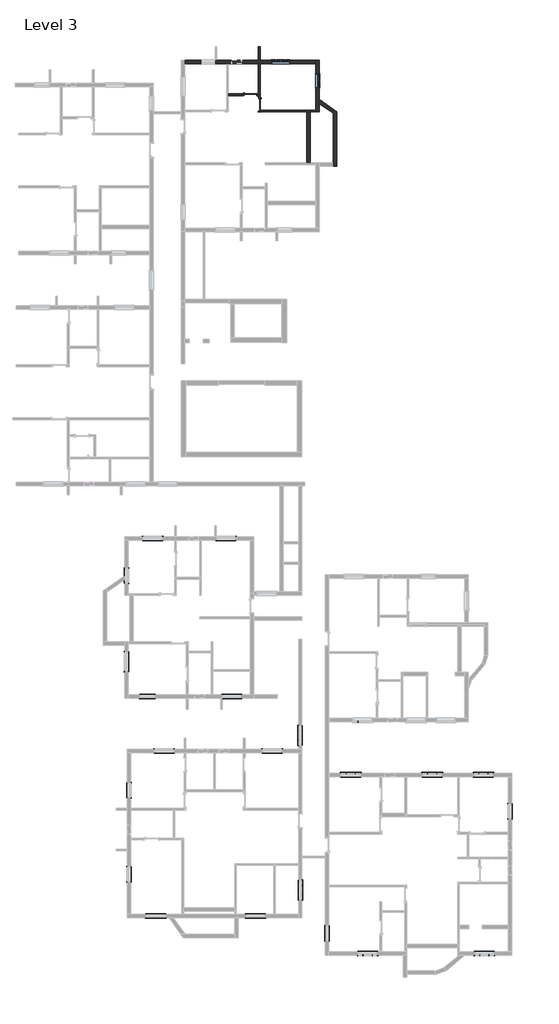
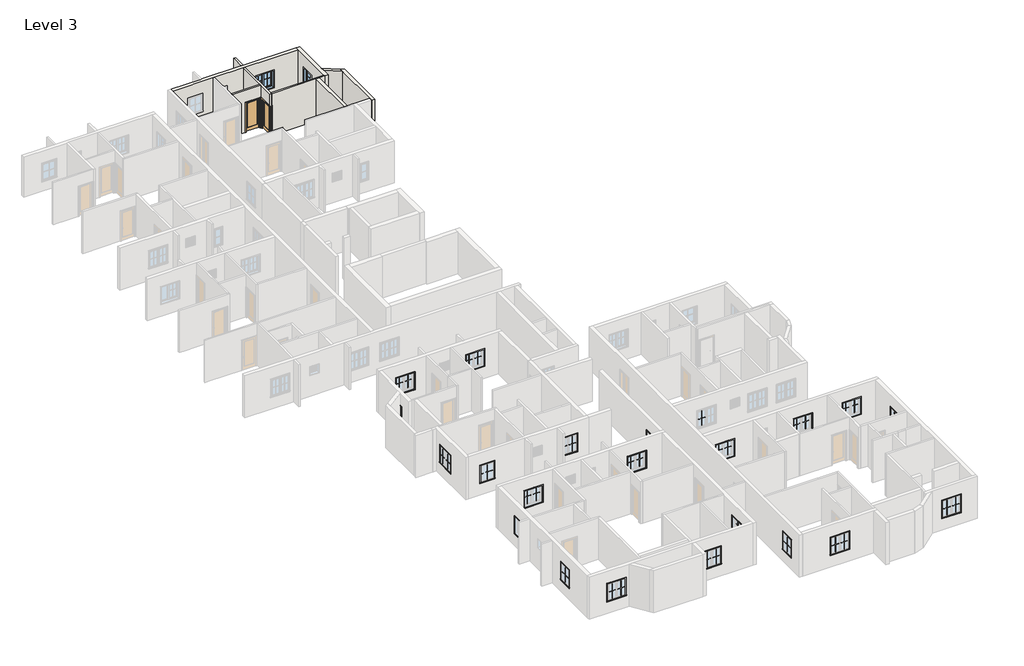
# One storey, part 6 of 7: 79 proxies, 9 walls, 2 doors, 2 windows.
"""IFC4 building model written with IfcOpenShell, lengths in millimetres."""

from ifc_helpers import new_model, si_unit, frame, origin, place, context, project, spatial, polyline, outline, extrude, faceted_brep, transform, mapped, element, save
from components import muntin_pattern_2x2_muntin_pattern_2x2_95b57395, muntin_pattern_2x2_muntin_pattern_2x2_4dfeb3f3, muntin_pattern_2x2_muntin_pattern_2x2_e852a7e4, trim_window_exterior_flat_with_sill_e4b28ec3, trim_window_exterior_flat_with_sill_7cfdd449, trim_window_interior_flat_picture_frame_39ff4276, trim_window_interior_flat_picture_frame_f1e0b15b, door_3c6ab76a, window_272f20d6, window_casement_double_4_x_4_af3140d2

model = new_model("IFC4")

# Units and contexts
model_context = context("Model", 3, world=origin())
ifc_project = project(units=[si_unit("LENGTHUNIT", "METRE", prefix="MILLI")], contexts=[model_context])

# Site, building, storey
site = spatial("IfcSite", under=ifc_project)
building = spatial("IfcBuilding", under=site)
storey = spatial("IfcBuildingStorey", under=building, Name="Level 3", Elevation=3200.4)

# Proxies
placement = place(None, origin())
muntin_pattern_2x2_muntin_pattern_2x2_shape = muntin_pattern_2x2_muntin_pattern_2x2_95b57395(model_context)
element("IfcBuildingElementProxy", 1, Name="Muntin Pattern_2x2 : Muntin Pattern_2x2", ObjectType="Muntin Pattern_2x2 : Muntin Pattern_2x2", at=placement, inside=storey, context=model_context, shape_type="MappedRepresentation", body=[
    mapped(muntin_pattern_2x2_muntin_pattern_2x2_shape, transform((17627.3240531, -20041.5997229, 4184.65), x_axis=(0.0, 1.0, 0.0), y_axis=(-1.0, 0.0, 0.0), z_axis=(0.0, 0.0, 1.0))),
])
element("IfcBuildingElementProxy", 2, Name="Muntin Pattern_2x2 : Muntin Pattern_2x2", ObjectType="Muntin Pattern_2x2 : Muntin Pattern_2x2", at=placement, inside=storey, context=model_context, shape_type="MappedRepresentation", body=[
    mapped(muntin_pattern_2x2_muntin_pattern_2x2_shape, transform((5625.8240531, -28048.9497229, 4184.65), x_axis=(0.0, 1.0, 0.0), y_axis=(-1.0, 0.0, 0.0), z_axis=(0.0, 0.0, 1.0))),
])
element("IfcBuildingElementProxy", 3, Name="Muntin Pattern_2x2 : Muntin Pattern_2x2", ObjectType="Muntin Pattern_2x2 : Muntin Pattern_2x2", at=placement, inside=storey, context=model_context, shape_type="MappedRepresentation", body=[
    mapped(muntin_pattern_2x2_muntin_pattern_2x2_shape, transform((-7378.9759469, -24172.9363256, 4184.65), x_axis=(0.0, 1.0, 0.0), y_axis=(-1.0, 0.0, 0.0), z_axis=(0.0, 0.0, 1.0))),
])
element("IfcBuildingElementProxy", 4, Name="Muntin Pattern_2x2 : Muntin Pattern_2x2", ObjectType="Muntin Pattern_2x2 : Muntin Pattern_2x2", at=placement, inside=storey, context=model_context, shape_type="MappedRepresentation", body=[
    mapped(muntin_pattern_2x2_muntin_pattern_2x2_shape, transform((-7169.4259469, -18656.0038828, 4184.65), x_axis=(0.0, -1.0, 0.0), y_axis=(1.0, 0.0, 0.0), z_axis=(0.0, 0.0, 1.0))),
])
element("IfcBuildingElementProxy", 5, Name="Muntin Pattern_2x2 : Muntin Pattern_2x2", ObjectType="Muntin Pattern_2x2 : Muntin Pattern_2x2", at=placement, inside=storey, context=model_context, shape_type="MappedRepresentation", body=[
    mapped(muntin_pattern_2x2_muntin_pattern_2x2_shape, transform((-6067.7009469, -12594.9288828, 4184.65), x_axis=(-1.0, 0.0, 0.0), y_axis=(0.0, -1.0, 0.0), z_axis=(0.0, 0.0, 1.0))),
])
element("IfcBuildingElementProxy", 6, Name="Muntin Pattern_2x2 : Muntin Pattern_2x2", ObjectType="Muntin Pattern_2x2 : Muntin Pattern_2x2", at=placement, inside=storey, context=model_context, shape_type="MappedRepresentation", body=[
    mapped(muntin_pattern_2x2_muntin_pattern_2x2_shape, transform((-7334.5259469, -4559.0038828, 4184.65), x_axis=(0.0, -1.0, 0.0), y_axis=(1.0, 0.0, 0.0), z_axis=(0.0, 0.0, 1.0))),
])
muntin_pattern_2x2_muntin_pattern_2x2_2_shape = muntin_pattern_2x2_muntin_pattern_2x2_4dfeb3f3(model_context)
element("IfcBuildingElementProxy", 7, Name="Muntin Pattern_2x2 : Muntin Pattern_2x2", ObjectType="Muntin Pattern_2x2 : Muntin Pattern_2x2", at=placement, inside=storey, context=model_context, shape_type="MappedRepresentation", body=[
    mapped(muntin_pattern_2x2_muntin_pattern_2x2_2_shape, transform((6976.7865531, -17530.1747229, 4184.65), x_axis=(1.0, 0.0, 0.0), y_axis=(0.0, 1.0, 0.0), z_axis=(0.0, 0.0, 1.0))),
])
element("IfcBuildingElementProxy", 8, Name="Muntin Pattern_2x2 : Muntin Pattern_2x2", ObjectType="Muntin Pattern_2x2 : Muntin Pattern_2x2", at=placement, inside=storey, context=model_context, shape_type="MappedRepresentation", body=[
    mapped(muntin_pattern_2x2_muntin_pattern_2x2_2_shape, transform((12323.4865531, -17530.1747229, 4184.65), x_axis=(1.0, 0.0, 0.0), y_axis=(0.0, 1.0, 0.0), z_axis=(0.0, 0.0, 1.0))),
])
element("IfcBuildingElementProxy", 9, Name="Muntin Pattern_2x2 : Muntin Pattern_2x2", ObjectType="Muntin Pattern_2x2 : Muntin Pattern_2x2", at=placement, inside=storey, context=model_context, shape_type="MappedRepresentation", body=[
    mapped(muntin_pattern_2x2_muntin_pattern_2x2_2_shape, transform((15682.6365531, -17530.1747229, 4184.65), x_axis=(1.0, 0.0, 0.0), y_axis=(0.0, 1.0, 0.0), z_axis=(0.0, 0.0, 1.0))),
])
element("IfcBuildingElementProxy", 10, Name="Muntin Pattern_2x2 : Muntin Pattern_2x2", ObjectType="Muntin Pattern_2x2 : Muntin Pattern_2x2", at=placement, inside=storey, context=model_context, shape_type="MappedRepresentation", body=[
    mapped(muntin_pattern_2x2_muntin_pattern_2x2_2_shape, transform((16349.3865531, -29474.5247229, 4184.65), x_axis=(-1.0, 0.0, 0.0), y_axis=(0.0, -1.0, 0.0), z_axis=(0.0, 0.0, 1.0))),
])
element("IfcBuildingElementProxy", 11, Name="Muntin Pattern_2x2 : Muntin Pattern_2x2", ObjectType="Muntin Pattern_2x2 : Muntin Pattern_2x2", at=placement, inside=storey, context=model_context, shape_type="MappedRepresentation", body=[
    mapped(muntin_pattern_2x2_muntin_pattern_2x2_2_shape, transform((8694.4615531, -29474.5247229, 4184.65), x_axis=(-1.0, 0.0, 0.0), y_axis=(0.0, -1.0, 0.0), z_axis=(0.0, 0.0, 1.0))),
])
element("IfcBuildingElementProxy", 12, Name="Muntin Pattern_2x2 : Muntin Pattern_2x2", ObjectType="Muntin Pattern_2x2 : Muntin Pattern_2x2", at=placement, inside=storey, context=model_context, shape_type="MappedRepresentation", body=[
    mapped(muntin_pattern_2x2_muntin_pattern_2x2_2_shape, transform((4070.0740531, -24902.8163828, 4184.65), x_axis=(0.0, -1.0, 0.0), y_axis=(1.0, 0.0, 0.0), z_axis=(0.0, 0.0, 1.0))),
])
element("IfcBuildingElementProxy", 13, Name="Muntin Pattern_2x2 : Muntin Pattern_2x2", ObjectType="Muntin Pattern_2x2 : Muntin Pattern_2x2", at=placement, inside=storey, context=model_context, shape_type="MappedRepresentation", body=[
    mapped(muntin_pattern_2x2_muntin_pattern_2x2_2_shape, transform((1325.2865531, -26996.7288828, 4184.65), x_axis=(-1.0, 0.0, 0.0), y_axis=(0.0, -1.0, 0.0), z_axis=(0.0, 0.0, 1.0))),
])
element("IfcBuildingElementProxy", 14, Name="Muntin Pattern_2x2 : Muntin Pattern_2x2", ObjectType="Muntin Pattern_2x2 : Muntin Pattern_2x2", at=placement, inside=storey, context=model_context, shape_type="MappedRepresentation", body=[
    mapped(muntin_pattern_2x2_muntin_pattern_2x2_2_shape, transform((-5208.8634469, -26996.7288828, 4184.65), x_axis=(-1.0, 0.0, 0.0), y_axis=(0.0, -1.0, 0.0), z_axis=(0.0, 0.0, 1.0))),
])
element("IfcBuildingElementProxy", 15, Name="Muntin Pattern_2x2 : Muntin Pattern_2x2", ObjectType="Muntin Pattern_2x2 : Muntin Pattern_2x2", at=placement, inside=storey, context=model_context, shape_type="MappedRepresentation", body=[
    mapped(muntin_pattern_2x2_muntin_pattern_2x2_2_shape, transform((1823.7615531, -15966.7788828, 4184.65), x_axis=(1.0, 0.0, 0.0), y_axis=(0.0, 1.0, 0.0), z_axis=(0.0, 0.0, 1.0))),
])
element("IfcBuildingElementProxy", 16, Name="Muntin Pattern_2x2 : Muntin Pattern_2x2", ObjectType="Muntin Pattern_2x2 : Muntin Pattern_2x2", at=placement, inside=storey, context=model_context, shape_type="MappedRepresentation", body=[
    mapped(muntin_pattern_2x2_muntin_pattern_2x2_2_shape, transform((-5272.3634469, -15966.7788828, 4184.65), x_axis=(1.0, 0.0, 0.0), y_axis=(0.0, 1.0, 0.0), z_axis=(0.0, 0.0, 1.0))),
])
element("IfcBuildingElementProxy", 17, Name="Muntin Pattern_2x2 : Muntin Pattern_2x2", ObjectType="Muntin Pattern_2x2 : Muntin Pattern_2x2", at=placement, inside=storey, context=model_context, shape_type="MappedRepresentation", body=[
    mapped(muntin_pattern_2x2_muntin_pattern_2x2_2_shape, transform((3860.5240531, -15358.7663828, 4184.65), x_axis=(0.0, 1.0, 0.0), y_axis=(-1.0, 0.0, 0.0), z_axis=(0.0, 0.0, 1.0))),
])
element("IfcBuildingElementProxy", 18, Name="Muntin Pattern_2x2 : Muntin Pattern_2x2", ObjectType="Muntin Pattern_2x2 : Muntin Pattern_2x2", at=placement, inside=storey, context=model_context, shape_type="MappedRepresentation", body=[
    mapped(muntin_pattern_2x2_muntin_pattern_2x2_2_shape, transform((-239.9884469, -12594.9288828, 4184.65), x_axis=(-1.0, 0.0, 0.0), y_axis=(0.0, -1.0, 0.0), z_axis=(0.0, 0.0, 1.0))),
])
element("IfcBuildingElementProxy", 19, Name="Muntin Pattern_2x2 : Muntin Pattern_2x2", ObjectType="Muntin Pattern_2x2 : Muntin Pattern_2x2", at=placement, inside=storey, context=model_context, shape_type="MappedRepresentation", body=[
    mapped(muntin_pattern_2x2_muntin_pattern_2x2_2_shape, transform((-7544.0759469, -10513.7163828, 4184.65), x_axis=(0.0, 1.0, 0.0), y_axis=(-1.0, 0.0, 0.0), z_axis=(0.0, 0.0, 1.0))),
])
element("IfcBuildingElementProxy", 20, Name="Muntin Pattern_2x2 : Muntin Pattern_2x2", ObjectType="Muntin Pattern_2x2 : Muntin Pattern_2x2", at=placement, inside=storey, context=model_context, shape_type="MappedRepresentation", body=[
    mapped(muntin_pattern_2x2_muntin_pattern_2x2_2_shape, transform((-6021.6634469, -2022.1788828, 4184.65), x_axis=(1.0, 0.0, 0.0), y_axis=(0.0, 1.0, 0.0), z_axis=(0.0, 0.0, 1.0))),
])
element("IfcBuildingElementProxy", 21, Name="Muntin Pattern_2x2 : Muntin Pattern_2x2", ObjectType="Muntin Pattern_2x2 : Muntin Pattern_2x2", at=placement, inside=storey, context=model_context, shape_type="MappedRepresentation", body=[
    mapped(muntin_pattern_2x2_muntin_pattern_2x2_2_shape, transform((-1221.0634469, -2022.1788828, 4184.65), x_axis=(1.0, 0.0, 0.0), y_axis=(0.0, 1.0, 0.0), z_axis=(0.0, 0.0, 1.0))),
])
muntin_pattern_2x2_muntin_pattern_2x2_3_shape = muntin_pattern_2x2_muntin_pattern_2x2_e852a7e4(model_context)
element("IfcBuildingElementProxy", 22, Name="Muntin Pattern_2x2 : Muntin Pattern_2x2", ObjectType="Muntin Pattern_2x2 : Muntin Pattern_2x2", at=placement, inside=storey, context=model_context, shape_type="MappedRepresentation", body=[
    mapped(muntin_pattern_2x2_muntin_pattern_2x2_3_shape, transform((7757.8365531, -14158.3247229, 4184.65), x_axis=(1.0, 0.0, 0.0), y_axis=(0.0, 1.0, 0.0), z_axis=(0.0, 0.0, 1.0))),
])
element("IfcBuildingElementProxy", 23, Name="Muntin Pattern_2x2 : Muntin Pattern_2x2", ObjectType="Muntin Pattern_2x2 : Muntin Pattern_2x2", at=placement, inside=storey, context=model_context, shape_type="MappedRepresentation", body=[
    mapped(muntin_pattern_2x2_muntin_pattern_2x2_3_shape, transform((7583.2115531, -17530.1747229, 4184.65), x_axis=(-1.0, 0.0, 0.0), y_axis=(0.0, -1.0, 0.0), z_axis=(0.0, 0.0, 1.0))),
])
element("IfcBuildingElementProxy", 24, Name="Muntin Pattern_2x2 : Muntin Pattern_2x2", ObjectType="Muntin Pattern_2x2 : Muntin Pattern_2x2", at=placement, inside=storey, context=model_context, shape_type="MappedRepresentation", body=[
    mapped(muntin_pattern_2x2_muntin_pattern_2x2_3_shape, transform((12929.9115531, -17530.1747229, 4184.65), x_axis=(-1.0, 0.0, 0.0), y_axis=(0.0, -1.0, 0.0), z_axis=(0.0, 0.0, 1.0))),
])
element("IfcBuildingElementProxy", 25, Name="Muntin Pattern_2x2 : Muntin Pattern_2x2", ObjectType="Muntin Pattern_2x2 : Muntin Pattern_2x2", at=placement, inside=storey, context=model_context, shape_type="MappedRepresentation", body=[
    mapped(muntin_pattern_2x2_muntin_pattern_2x2_3_shape, transform((16289.0615531, -17530.1747229, 4184.65), x_axis=(-1.0, 0.0, 0.0), y_axis=(0.0, -1.0, 0.0), z_axis=(0.0, 0.0, 1.0))),
])
element("IfcBuildingElementProxy", 26, Name="Muntin Pattern_2x2 : Muntin Pattern_2x2", ObjectType="Muntin Pattern_2x2 : Muntin Pattern_2x2", at=placement, inside=storey, context=model_context, shape_type="MappedRepresentation", body=[
    mapped(muntin_pattern_2x2_muntin_pattern_2x2_3_shape, transform((15742.9615531, -29474.5247229, 4184.65), x_axis=(1.0, 0.0, 0.0), y_axis=(0.0, 1.0, 0.0), z_axis=(0.0, 0.0, 1.0))),
])
element("IfcBuildingElementProxy", 27, Name="Muntin Pattern_2x2 : Muntin Pattern_2x2", ObjectType="Muntin Pattern_2x2 : Muntin Pattern_2x2", at=placement, inside=storey, context=model_context, shape_type="MappedRepresentation", body=[
    mapped(muntin_pattern_2x2_muntin_pattern_2x2_3_shape, transform((8088.0365531, -29474.5247229, 4184.65), x_axis=(1.0, 0.0, 0.0), y_axis=(0.0, 1.0, 0.0), z_axis=(0.0, 0.0, 1.0))),
])
element("IfcBuildingElementProxy", 28, Name="Muntin Pattern_2x2 : Muntin Pattern_2x2", ObjectType="Muntin Pattern_2x2 : Muntin Pattern_2x2", at=placement, inside=storey, context=model_context, shape_type="MappedRepresentation", body=[
    mapped(muntin_pattern_2x2_muntin_pattern_2x2_3_shape, transform((4070.0740531, -25509.2413828, 4184.65), x_axis=(0.0, 1.0, 0.0), y_axis=(-1.0, 0.0, 0.0), z_axis=(0.0, 0.0, 1.0))),
])
element("IfcBuildingElementProxy", 29, Name="Muntin Pattern_2x2 : Muntin Pattern_2x2", ObjectType="Muntin Pattern_2x2 : Muntin Pattern_2x2", at=placement, inside=storey, context=model_context, shape_type="MappedRepresentation", body=[
    mapped(muntin_pattern_2x2_muntin_pattern_2x2_3_shape, transform((718.8615531, -26996.7288828, 4184.65), x_axis=(1.0, 0.0, 0.0), y_axis=(0.0, 1.0, 0.0), z_axis=(0.0, 0.0, 1.0))),
])
element("IfcBuildingElementProxy", 30, Name="Muntin Pattern_2x2 : Muntin Pattern_2x2", ObjectType="Muntin Pattern_2x2 : Muntin Pattern_2x2", at=placement, inside=storey, context=model_context, shape_type="MappedRepresentation", body=[
    mapped(muntin_pattern_2x2_muntin_pattern_2x2_3_shape, transform((-5815.2884469, -26996.7288828, 4184.65), x_axis=(1.0, 0.0, 0.0), y_axis=(0.0, 1.0, 0.0), z_axis=(0.0, 0.0, 1.0))),
])
element("IfcBuildingElementProxy", 31, Name="Muntin Pattern_2x2 : Muntin Pattern_2x2", ObjectType="Muntin Pattern_2x2 : Muntin Pattern_2x2", at=placement, inside=storey, context=model_context, shape_type="MappedRepresentation", body=[
    mapped(muntin_pattern_2x2_muntin_pattern_2x2_3_shape, transform((2430.1865531, -15966.7788828, 4184.65), x_axis=(-1.0, 0.0, 0.0), y_axis=(0.0, -1.0, 0.0), z_axis=(0.0, 0.0, 1.0))),
])
element("IfcBuildingElementProxy", 32, Name="Muntin Pattern_2x2 : Muntin Pattern_2x2", ObjectType="Muntin Pattern_2x2 : Muntin Pattern_2x2", at=placement, inside=storey, context=model_context, shape_type="MappedRepresentation", body=[
    mapped(muntin_pattern_2x2_muntin_pattern_2x2_3_shape, transform((-4665.9384469, -15966.7788828, 4184.65), x_axis=(-1.0, 0.0, 0.0), y_axis=(0.0, -1.0, 0.0), z_axis=(0.0, 0.0, 1.0))),
])
element("IfcBuildingElementProxy", 33, Name="Muntin Pattern_2x2 : Muntin Pattern_2x2", ObjectType="Muntin Pattern_2x2 : Muntin Pattern_2x2", at=placement, inside=storey, context=model_context, shape_type="MappedRepresentation", body=[
    mapped(muntin_pattern_2x2_muntin_pattern_2x2_3_shape, transform((3860.5240531, -14752.3413828, 4184.65), x_axis=(0.0, -1.0, 0.0), y_axis=(1.0, 0.0, 0.0), z_axis=(0.0, 0.0, 1.0))),
])
element("IfcBuildingElementProxy", 34, Name="Muntin Pattern_2x2 : Muntin Pattern_2x2", ObjectType="Muntin Pattern_2x2 : Muntin Pattern_2x2", at=placement, inside=storey, context=model_context, shape_type="MappedRepresentation", body=[
    mapped(muntin_pattern_2x2_muntin_pattern_2x2_3_shape, transform((-846.4134469, -12594.9288828, 4184.65), x_axis=(1.0, 0.0, 0.0), y_axis=(0.0, 1.0, 0.0), z_axis=(0.0, 0.0, 1.0))),
])
element("IfcBuildingElementProxy", 35, Name="Muntin Pattern_2x2 : Muntin Pattern_2x2", ObjectType="Muntin Pattern_2x2 : Muntin Pattern_2x2", at=placement, inside=storey, context=model_context, shape_type="MappedRepresentation", body=[
    mapped(muntin_pattern_2x2_muntin_pattern_2x2_3_shape, transform((-7544.0759469, -9907.2913828, 4184.65), x_axis=(0.0, -1.0, 0.0), y_axis=(1.0, 0.0, 0.0), z_axis=(0.0, 0.0, 1.0))),
])
element("IfcBuildingElementProxy", 36, Name="Muntin Pattern_2x2 : Muntin Pattern_2x2", ObjectType="Muntin Pattern_2x2 : Muntin Pattern_2x2", at=placement, inside=storey, context=model_context, shape_type="MappedRepresentation", body=[
    mapped(muntin_pattern_2x2_muntin_pattern_2x2_3_shape, transform((-5415.2384469, -2022.1788828, 4184.65), x_axis=(-1.0, 0.0, 0.0), y_axis=(0.0, -1.0, 0.0), z_axis=(0.0, 0.0, 1.0))),
])
element("IfcBuildingElementProxy", 37, Name="Muntin Pattern_2x2 : Muntin Pattern_2x2", ObjectType="Muntin Pattern_2x2 : Muntin Pattern_2x2", at=placement, inside=storey, context=model_context, shape_type="MappedRepresentation", body=[
    mapped(muntin_pattern_2x2_muntin_pattern_2x2_3_shape, transform((-614.6384469, -2022.1788828, 4184.65), x_axis=(-1.0, 0.0, 0.0), y_axis=(0.0, -1.0, 0.0), z_axis=(0.0, 0.0, 1.0))),
])
trim_window_exterior_flat_with_sill_shape = trim_window_exterior_flat_with_sill_e4b28ec3(model_context)
element("IfcBuildingElementProxy", 38, Name="Trim-Window-Exterior-Flat : with Sill", ObjectType="Trim-Window-Exterior-Flat : with Sill", at=placement, inside=storey, context=model_context, shape_type="MappedRepresentation", body=[
    mapped(trim_window_exterior_flat_with_sill_shape, transform((17617.7990531, -20041.5997229, 5334.0), x_axis=(0.0, -1.0, 0.0), y_axis=(0.0, 0.0, 1.0), z_axis=(-1.0, 0.0, 0.0))),
])
element("IfcBuildingElementProxy", 39, Name="Trim-Window-Exterior-Flat : with Sill", ObjectType="Trim-Window-Exterior-Flat : with Sill", at=placement, inside=storey, context=model_context, shape_type="MappedRepresentation", body=[
    mapped(trim_window_exterior_flat_with_sill_shape, transform((5616.2990531, -28048.9497229, 5334.0), x_axis=(0.0, -1.0, 0.0), y_axis=(0.0, 0.0, 1.0), z_axis=(-1.0, 0.0, 0.0))),
])
element("IfcBuildingElementProxy", 40, Name="Trim-Window-Exterior-Flat : with Sill", ObjectType="Trim-Window-Exterior-Flat : with Sill", at=placement, inside=storey, context=model_context, shape_type="MappedRepresentation", body=[
    mapped(trim_window_exterior_flat_with_sill_shape, transform((-7388.5009469, -24172.9363256, 5334.0), x_axis=(0.0, -1.0, 0.0), y_axis=(0.0, 0.0, 1.0), z_axis=(-1.0, 0.0, 0.0))),
])
element("IfcBuildingElementProxy", 41, Name="Trim-Window-Exterior-Flat : with Sill", ObjectType="Trim-Window-Exterior-Flat : with Sill", at=placement, inside=storey, context=model_context, shape_type="MappedRepresentation", body=[
    mapped(trim_window_exterior_flat_with_sill_shape, transform((-7159.9009469, -18656.0038828, 5334.0), x_axis=(0.0, 1.0, 0.0), y_axis=(0.0, 0.0, 1.0), z_axis=(1.0, 0.0, 0.0))),
])
element("IfcBuildingElementProxy", 42, Name="Trim-Window-Exterior-Flat : with Sill", ObjectType="Trim-Window-Exterior-Flat : with Sill", at=placement, inside=storey, context=model_context, shape_type="MappedRepresentation", body=[
    mapped(trim_window_exterior_flat_with_sill_shape, transform((-6067.7009469, -12604.4538828, 5334.0), x_axis=(1.0, 0.0, 0.0), y_axis=(0.0, 0.0, 1.0), z_axis=(0.0, -1.0, 0.0))),
])
element("IfcBuildingElementProxy", 43, Name="Trim-Window-Exterior-Flat : with Sill", ObjectType="Trim-Window-Exterior-Flat : with Sill", at=placement, inside=storey, context=model_context, shape_type="MappedRepresentation", body=[
    mapped(trim_window_exterior_flat_with_sill_shape, transform((-7325.0009469, -4559.0038828, 5334.0), x_axis=(0.0, 1.0, 0.0), y_axis=(0.0, 0.0, 1.0), z_axis=(1.0, 0.0, 0.0))),
])
trim_window_exterior_flat_with_sill_2_shape = trim_window_exterior_flat_with_sill_7cfdd449(model_context)
element("IfcBuildingElementProxy", 44, Name="Trim-Window-Exterior-Flat : with Sill", ObjectType="Trim-Window-Exterior-Flat : with Sill", at=placement, inside=storey, context=model_context, shape_type="MappedRepresentation", body=[
    mapped(trim_window_exterior_flat_with_sill_2_shape, transform((7279.9990531, -17520.6497229, 5334.0), x_axis=(-1.0, 0.0, 0.0), y_axis=(0.0, 0.0, 1.0), z_axis=(0.0, 1.0, 0.0))),
])
element("IfcBuildingElementProxy", 45, Name="Trim-Window-Exterior-Flat : with Sill", ObjectType="Trim-Window-Exterior-Flat : with Sill", at=placement, inside=storey, context=model_context, shape_type="MappedRepresentation", body=[
    mapped(trim_window_exterior_flat_with_sill_2_shape, transform((12626.6990531, -17520.6497229, 5334.0), x_axis=(-1.0, 0.0, 0.0), y_axis=(0.0, 0.0, 1.0), z_axis=(0.0, 1.0, 0.0))),
])
element("IfcBuildingElementProxy", 46, Name="Trim-Window-Exterior-Flat : with Sill", ObjectType="Trim-Window-Exterior-Flat : with Sill", at=placement, inside=storey, context=model_context, shape_type="MappedRepresentation", body=[
    mapped(trim_window_exterior_flat_with_sill_2_shape, transform((15985.8490531, -17520.6497229, 5334.0), x_axis=(-1.0, 0.0, 0.0), y_axis=(0.0, 0.0, 1.0), z_axis=(0.0, 1.0, 0.0))),
])
element("IfcBuildingElementProxy", 47, Name="Trim-Window-Exterior-Flat : with Sill", ObjectType="Trim-Window-Exterior-Flat : with Sill", at=placement, inside=storey, context=model_context, shape_type="MappedRepresentation", body=[
    mapped(trim_window_exterior_flat_with_sill_2_shape, transform((16046.1740531, -29484.0497229, 5334.0), x_axis=(1.0, 0.0, 0.0), y_axis=(0.0, 0.0, 1.0), z_axis=(0.0, -1.0, 0.0))),
])
element("IfcBuildingElementProxy", 48, Name="Trim-Window-Exterior-Flat : with Sill", ObjectType="Trim-Window-Exterior-Flat : with Sill", at=placement, inside=storey, context=model_context, shape_type="MappedRepresentation", body=[
    mapped(trim_window_exterior_flat_with_sill_2_shape, transform((8391.2490531, -29484.0497229, 5334.0), x_axis=(1.0, 0.0, 0.0), y_axis=(0.0, 0.0, 1.0), z_axis=(0.0, -1.0, 0.0))),
])
element("IfcBuildingElementProxy", 49, Name="Trim-Window-Exterior-Flat : with Sill", ObjectType="Trim-Window-Exterior-Flat : with Sill", at=placement, inside=storey, context=model_context, shape_type="MappedRepresentation", body=[
    mapped(trim_window_exterior_flat_with_sill_2_shape, transform((4079.5990531, -25206.0288828, 5334.0), x_axis=(0.0, 1.0, 0.0), y_axis=(0.0, 0.0, 1.0), z_axis=(1.0, 0.0, 0.0))),
])
element("IfcBuildingElementProxy", 50, Name="Trim-Window-Exterior-Flat : with Sill", ObjectType="Trim-Window-Exterior-Flat : with Sill", at=placement, inside=storey, context=model_context, shape_type="MappedRepresentation", body=[
    mapped(trim_window_exterior_flat_with_sill_2_shape, transform((1022.0740531, -27006.2538828, 5334.0), x_axis=(1.0, 0.0, 0.0), y_axis=(0.0, 0.0, 1.0), z_axis=(0.0, -1.0, 0.0))),
])
element("IfcBuildingElementProxy", 51, Name="Trim-Window-Exterior-Flat : with Sill", ObjectType="Trim-Window-Exterior-Flat : with Sill", at=placement, inside=storey, context=model_context, shape_type="MappedRepresentation", body=[
    mapped(trim_window_exterior_flat_with_sill_2_shape, transform((-5512.0759469, -27006.2538828, 5334.0), x_axis=(1.0, 0.0, 0.0), y_axis=(0.0, 0.0, 1.0), z_axis=(0.0, -1.0, 0.0))),
])
element("IfcBuildingElementProxy", 52, Name="Trim-Window-Exterior-Flat : with Sill", ObjectType="Trim-Window-Exterior-Flat : with Sill", at=placement, inside=storey, context=model_context, shape_type="MappedRepresentation", body=[
    mapped(trim_window_exterior_flat_with_sill_2_shape, transform((2126.9740531, -15957.2538828, 5334.0), x_axis=(-1.0, 0.0, 0.0), y_axis=(0.0, 0.0, 1.0), z_axis=(0.0, 1.0, 0.0))),
])
element("IfcBuildingElementProxy", 53, Name="Trim-Window-Exterior-Flat : with Sill", ObjectType="Trim-Window-Exterior-Flat : with Sill", at=placement, inside=storey, context=model_context, shape_type="MappedRepresentation", body=[
    mapped(trim_window_exterior_flat_with_sill_2_shape, transform((-4969.1509469, -15957.2538828, 5334.0), x_axis=(-1.0, 0.0, 0.0), y_axis=(0.0, 0.0, 1.0), z_axis=(0.0, 1.0, 0.0))),
])
element("IfcBuildingElementProxy", 54, Name="Trim-Window-Exterior-Flat : with Sill", ObjectType="Trim-Window-Exterior-Flat : with Sill", at=placement, inside=storey, context=model_context, shape_type="MappedRepresentation", body=[
    mapped(trim_window_exterior_flat_with_sill_2_shape, transform((3850.9990531, -15055.5538828, 5334.0), x_axis=(0.0, -1.0, 0.0), y_axis=(0.0, 0.0, 1.0), z_axis=(-1.0, 0.0, 0.0))),
])
element("IfcBuildingElementProxy", 55, Name="Trim-Window-Exterior-Flat : with Sill", ObjectType="Trim-Window-Exterior-Flat : with Sill", at=placement, inside=storey, context=model_context, shape_type="MappedRepresentation", body=[
    mapped(trim_window_exterior_flat_with_sill_2_shape, transform((-543.2009469, -12604.4538828, 5334.0), x_axis=(1.0, 0.0, 0.0), y_axis=(0.0, 0.0, 1.0), z_axis=(0.0, -1.0, 0.0))),
])
element("IfcBuildingElementProxy", 56, Name="Trim-Window-Exterior-Flat : with Sill", ObjectType="Trim-Window-Exterior-Flat : with Sill", at=placement, inside=storey, context=model_context, shape_type="MappedRepresentation", body=[
    mapped(trim_window_exterior_flat_with_sill_2_shape, transform((-7553.6009469, -10210.5038828, 5334.0), x_axis=(0.0, -1.0, 0.0), y_axis=(0.0, 0.0, 1.0), z_axis=(-1.0, 0.0, 0.0))),
])
element("IfcBuildingElementProxy", 57, Name="Trim-Window-Exterior-Flat : with Sill", ObjectType="Trim-Window-Exterior-Flat : with Sill", at=placement, inside=storey, context=model_context, shape_type="MappedRepresentation", body=[
    mapped(trim_window_exterior_flat_with_sill_2_shape, transform((-5718.4509469, -2012.6538828, 5334.0), x_axis=(-1.0, 0.0, 0.0), y_axis=(0.0, 0.0, 1.0), z_axis=(0.0, 1.0, 0.0))),
])
element("IfcBuildingElementProxy", 58, Name="Trim-Window-Exterior-Flat : with Sill", ObjectType="Trim-Window-Exterior-Flat : with Sill", at=placement, inside=storey, context=model_context, shape_type="MappedRepresentation", body=[
    mapped(trim_window_exterior_flat_with_sill_2_shape, transform((-917.8509469, -2012.6538828, 5334.0), x_axis=(-1.0, 0.0, 0.0), y_axis=(0.0, 0.0, 1.0), z_axis=(0.0, 1.0, 0.0))),
])
trim_window_interior_flat_picture_frame_shape = trim_window_interior_flat_picture_frame_39ff4276(model_context)
element("IfcBuildingElementProxy", 59, Name="Trim-Window-Interior-Flat : Picture Frame", ObjectType="Trim-Window-Interior-Flat : Picture Frame", at=placement, inside=storey, context=model_context, shape_type="MappedRepresentation", body=[
    mapped(trim_window_interior_flat_picture_frame_shape, transform((17846.3990531, -20041.5997229, 5334.0), x_axis=(0.0, 1.0, 0.0), y_axis=(0.0, 0.0, 1.0), z_axis=(1.0, 0.0, 0.0))),
])
element("IfcBuildingElementProxy", 60, Name="Trim-Window-Interior-Flat : Picture Frame", ObjectType="Trim-Window-Interior-Flat : Picture Frame", at=placement, inside=storey, context=model_context, shape_type="MappedRepresentation", body=[
    mapped(trim_window_interior_flat_picture_frame_shape, transform((5844.8990531, -28048.9497229, 5334.0), x_axis=(0.0, 1.0, 0.0), y_axis=(0.0, 0.0, 1.0), z_axis=(1.0, 0.0, 0.0))),
])
element("IfcBuildingElementProxy", 61, Name="Trim-Window-Interior-Flat : Picture Frame", ObjectType="Trim-Window-Interior-Flat : Picture Frame", at=placement, inside=storey, context=model_context, shape_type="MappedRepresentation", body=[
    mapped(trim_window_interior_flat_picture_frame_shape, transform((-7159.9009469, -24172.9363256, 5334.0), x_axis=(0.0, 1.0, 0.0), y_axis=(0.0, 0.0, 1.0), z_axis=(1.0, 0.0, 0.0))),
])
element("IfcBuildingElementProxy", 62, Name="Trim-Window-Interior-Flat : Picture Frame", ObjectType="Trim-Window-Interior-Flat : Picture Frame", at=placement, inside=storey, context=model_context, shape_type="MappedRepresentation", body=[
    mapped(trim_window_interior_flat_picture_frame_shape, transform((-7388.5009469, -18656.0038828, 5334.0), x_axis=(0.0, -1.0, 0.0), y_axis=(0.0, 0.0, 1.0), z_axis=(-1.0, 0.0, 0.0))),
])
element("IfcBuildingElementProxy", 63, Name="Trim-Window-Interior-Flat : Picture Frame", ObjectType="Trim-Window-Interior-Flat : Picture Frame", at=placement, inside=storey, context=model_context, shape_type="MappedRepresentation", body=[
    mapped(trim_window_interior_flat_picture_frame_shape, transform((-6067.7009469, -12375.8538828, 5334.0), x_axis=(-1.0, 0.0, 0.0), y_axis=(0.0, 0.0, 1.0), z_axis=(0.0, 1.0, 0.0))),
])
element("IfcBuildingElementProxy", 64, Name="Trim-Window-Interior-Flat : Picture Frame", ObjectType="Trim-Window-Interior-Flat : Picture Frame", at=placement, inside=storey, context=model_context, shape_type="MappedRepresentation", body=[
    mapped(trim_window_interior_flat_picture_frame_shape, transform((-7553.6009469, -4559.0038828, 5334.0), x_axis=(0.0, -1.0, 0.0), y_axis=(0.0, 0.0, 1.0), z_axis=(-1.0, 0.0, 0.0))),
])
trim_window_interior_flat_picture_frame_2_shape = trim_window_interior_flat_picture_frame_f1e0b15b(model_context)
element("IfcBuildingElementProxy", 65, Name="Trim-Window-Interior-Flat : Picture Frame", ObjectType="Trim-Window-Interior-Flat : Picture Frame", at=placement, inside=storey, context=model_context, shape_type="MappedRepresentation", body=[
    mapped(trim_window_interior_flat_picture_frame_2_shape, transform((7279.9990531, -17749.2497229, 5334.0), x_axis=(1.0, 0.0, 0.0), y_axis=(0.0, 0.0, 1.0), z_axis=(0.0, -1.0, 0.0))),
])
element("IfcBuildingElementProxy", 66, Name="Trim-Window-Interior-Flat : Picture Frame", ObjectType="Trim-Window-Interior-Flat : Picture Frame", at=placement, inside=storey, context=model_context, shape_type="MappedRepresentation", body=[
    mapped(trim_window_interior_flat_picture_frame_2_shape, transform((12626.6990531, -17749.2497229, 5334.0), x_axis=(1.0, 0.0, 0.0), y_axis=(0.0, 0.0, 1.0), z_axis=(0.0, -1.0, 0.0))),
])
element("IfcBuildingElementProxy", 67, Name="Trim-Window-Interior-Flat : Picture Frame", ObjectType="Trim-Window-Interior-Flat : Picture Frame", at=placement, inside=storey, context=model_context, shape_type="MappedRepresentation", body=[
    mapped(trim_window_interior_flat_picture_frame_2_shape, transform((15985.8490531, -17749.2497229, 5334.0), x_axis=(1.0, 0.0, 0.0), y_axis=(0.0, 0.0, 1.0), z_axis=(0.0, -1.0, 0.0))),
])
element("IfcBuildingElementProxy", 68, Name="Trim-Window-Interior-Flat : Picture Frame", ObjectType="Trim-Window-Interior-Flat : Picture Frame", at=placement, inside=storey, context=model_context, shape_type="MappedRepresentation", body=[
    mapped(trim_window_interior_flat_picture_frame_2_shape, transform((16046.1740531, -29255.4497229, 5334.0), x_axis=(-1.0, 0.0, 0.0), y_axis=(0.0, 0.0, 1.0), z_axis=(0.0, 1.0, 0.0))),
])
element("IfcBuildingElementProxy", 69, Name="Trim-Window-Interior-Flat : Picture Frame", ObjectType="Trim-Window-Interior-Flat : Picture Frame", at=placement, inside=storey, context=model_context, shape_type="MappedRepresentation", body=[
    mapped(trim_window_interior_flat_picture_frame_2_shape, transform((8391.2490531, -29255.4497229, 5334.0), x_axis=(-1.0, 0.0, 0.0), y_axis=(0.0, 0.0, 1.0), z_axis=(0.0, 1.0, 0.0))),
])
element("IfcBuildingElementProxy", 70, Name="Trim-Window-Interior-Flat : Picture Frame", ObjectType="Trim-Window-Interior-Flat : Picture Frame", at=placement, inside=storey, context=model_context, shape_type="MappedRepresentation", body=[
    mapped(trim_window_interior_flat_picture_frame_2_shape, transform((3850.9990531, -25206.0288828, 5334.0), x_axis=(0.0, -1.0, 0.0), y_axis=(0.0, 0.0, 1.0), z_axis=(-1.0, 0.0, 0.0))),
])
element("IfcBuildingElementProxy", 71, Name="Trim-Window-Interior-Flat : Picture Frame", ObjectType="Trim-Window-Interior-Flat : Picture Frame", at=placement, inside=storey, context=model_context, shape_type="MappedRepresentation", body=[
    mapped(trim_window_interior_flat_picture_frame_2_shape, transform((1022.0740531, -26777.6538828, 5334.0), x_axis=(-1.0, 0.0, 0.0), y_axis=(0.0, 0.0, 1.0), z_axis=(0.0, 1.0, 0.0))),
])
element("IfcBuildingElementProxy", 72, Name="Trim-Window-Interior-Flat : Picture Frame", ObjectType="Trim-Window-Interior-Flat : Picture Frame", at=placement, inside=storey, context=model_context, shape_type="MappedRepresentation", body=[
    mapped(trim_window_interior_flat_picture_frame_2_shape, transform((-5512.0759469, -26777.6538828, 5334.0), x_axis=(-1.0, 0.0, 0.0), y_axis=(0.0, 0.0, 1.0), z_axis=(0.0, 1.0, 0.0))),
])
element("IfcBuildingElementProxy", 73, Name="Trim-Window-Interior-Flat : Picture Frame", ObjectType="Trim-Window-Interior-Flat : Picture Frame", at=placement, inside=storey, context=model_context, shape_type="MappedRepresentation", body=[
    mapped(trim_window_interior_flat_picture_frame_2_shape, transform((2126.9740531, -16185.8538828, 5334.0), x_axis=(1.0, 0.0, 0.0), y_axis=(0.0, 0.0, 1.0), z_axis=(0.0, -1.0, 0.0))),
])
element("IfcBuildingElementProxy", 74, Name="Trim-Window-Interior-Flat : Picture Frame", ObjectType="Trim-Window-Interior-Flat : Picture Frame", at=placement, inside=storey, context=model_context, shape_type="MappedRepresentation", body=[
    mapped(trim_window_interior_flat_picture_frame_2_shape, transform((-4969.1509469, -16185.8538828, 5334.0), x_axis=(1.0, 0.0, 0.0), y_axis=(0.0, 0.0, 1.0), z_axis=(0.0, -1.0, 0.0))),
])
element("IfcBuildingElementProxy", 75, Name="Trim-Window-Interior-Flat : Picture Frame", ObjectType="Trim-Window-Interior-Flat : Picture Frame", at=placement, inside=storey, context=model_context, shape_type="MappedRepresentation", body=[
    mapped(trim_window_interior_flat_picture_frame_2_shape, transform((4079.5990531, -15055.5538828, 5334.0), x_axis=(0.0, 1.0, 0.0), y_axis=(0.0, 0.0, 1.0), z_axis=(1.0, 0.0, 0.0))),
])
element("IfcBuildingElementProxy", 76, Name="Trim-Window-Interior-Flat : Picture Frame", ObjectType="Trim-Window-Interior-Flat : Picture Frame", at=placement, inside=storey, context=model_context, shape_type="MappedRepresentation", body=[
    mapped(trim_window_interior_flat_picture_frame_2_shape, transform((-543.2009469, -12375.8538828, 5334.0), x_axis=(-1.0, 0.0, 0.0), y_axis=(0.0, 0.0, 1.0), z_axis=(0.0, 1.0, 0.0))),
])
element("IfcBuildingElementProxy", 77, Name="Trim-Window-Interior-Flat : Picture Frame", ObjectType="Trim-Window-Interior-Flat : Picture Frame", at=placement, inside=storey, context=model_context, shape_type="MappedRepresentation", body=[
    mapped(trim_window_interior_flat_picture_frame_2_shape, transform((-7325.0009469, -10210.5038828, 5334.0), x_axis=(0.0, 1.0, 0.0), y_axis=(0.0, 0.0, 1.0), z_axis=(1.0, 0.0, 0.0))),
])
element("IfcBuildingElementProxy", 78, Name="Trim-Window-Interior-Flat : Picture Frame", ObjectType="Trim-Window-Interior-Flat : Picture Frame", at=placement, inside=storey, context=model_context, shape_type="MappedRepresentation", body=[
    mapped(trim_window_interior_flat_picture_frame_2_shape, transform((-5718.4509469, -2241.2538828, 5334.0), x_axis=(1.0, 0.0, 0.0), y_axis=(0.0, 0.0, 1.0), z_axis=(0.0, -1.0, 0.0))),
])
element("IfcBuildingElementProxy", 79, Name="Trim-Window-Interior-Flat : Picture Frame", ObjectType="Trim-Window-Interior-Flat : Picture Frame", at=placement, inside=storey, context=model_context, shape_type="MappedRepresentation", body=[
    mapped(trim_window_interior_flat_picture_frame_2_shape, transform((-917.8509469, -2241.2538828, 5334.0), x_axis=(1.0, 0.0, 0.0), y_axis=(0.0, 0.0, 1.0), z_axis=(0.0, -1.0, 0.0))),
])

# Doors
door_shape = door_3c6ab76a(model_context)
element("IfcDoor", 80, ObjectType="Door-Interior-Single-1_Panel-Wood : 2'6\" x 7' door", at=placement, inside=storey, context=model_context, shape_type="MappedRepresentation", body=[
    mapped(door_shape, transform((669.6490531, 27005.8505084, 3200.4), x_axis=(1.0, 0.0, 0.0), y_axis=(0.0, 1.0, 0.0), z_axis=(0.0, 0.0, 1.0))),
])
element("IfcDoor", 81, ObjectType="Door-Interior-Single-1_Panel-Wood : 36\" x 84\"", at=placement, inside=storey, context=model_context, shape_type="MappedRepresentation", body=[
    mapped(door_shape, transform((1282.4240531, 26367.6755084, 3200.4), x_axis=(0.0, -1.0, 0.0), y_axis=(1.0, 0.0, 0.0), z_axis=(0.0, 0.0, 1.0))),
])

# Walls
element("IfcWall", 82, ObjectType="4.5\" wall", at=placement, inside=storey, context=model_context, shape_type="Brep", body=[
    faceted_brep([(1336.3990531, 29041.0255084, 6248.4), (1336.3990531, 25993.0255084, 6248.4), (1336.3990531, 25878.7255084, 6248.4), (1336.3990531, 25878.7255084, 3200.4), (1336.3990531, 25885.0755084, 3200.4), (1336.3990531, 25885.0755084, 5359.4), (1336.3990531, 26850.2755084, 5359.4), (1336.3990531, 26850.2755084, 3200.4), (1336.3990531, 29041.0255084, 3200.4), (1222.0990531, 25878.7255084, 6248.4), (1222.0990531, 26945.5255084, 6248.4), (1222.0990531, 27059.8255084, 6248.4), (1222.0990531, 29041.0255084, 6248.4), (1222.0990531, 29041.0255084, 3200.4), (1222.0990531, 27059.8255084, 3200.4), (1222.0990531, 26945.5255084, 3200.4), (1222.0990531, 26850.2755084, 3200.4), (1222.0990531, 26850.2755084, 5359.4), (1222.0990531, 25885.0755084, 5359.4), (1222.0990531, 25885.0755084, 3200.4), (1222.0990531, 25878.7255084, 3200.4)], [[[0, 1, 2, 3, 4, 5, 6, 7, 8]], [[9, 10, 11, 12, 13, 14, 15, 16, 17, 18, 19, 20]], [[13, 8, 7, 16, 15, 14]], [[3, 20, 19, 4]], [[2, 1, 0, 12, 11, 10, 9]], [[0, 8, 13, 12]], [[3, 2, 9, 20]], [[18, 5, 4, 19]], [[5, 18, 17, 6]], [[6, 17, 16, 7]]]),
])
element("IfcWall", 83, ObjectType="4.5\" wall", at=placement, inside=storey, context=model_context, shape_type="SweptSolid", body=[
    extrude(outline(polyline([(6248.4, 1222.0990531), (6248.4, -759.1009469), (3200.4, -759.1009469), (3200.4, 187.0490531), (5359.4, 187.0490531), (5359.4, 1152.2490531), (3200.4, 1152.2490531), (3200.4, 1222.0990531), (6248.4, 1222.0990531)])), frame((0.0, 26945.5255084, 0.0), z_axis=(0.0, 1.0, 0.0), x_axis=(0.0, 0.0, 1.0)), (0.0, 0.0, 1.0), 114.3),
])
element("IfcWall", 84, ObjectType="4.5\" wall", at=placement, inside=storey, context=model_context, shape_type="Brep", body=[
    faceted_brep([(4993.9990531, 25993.0255084, 3200.4), (1336.3990531, 25993.0255084, 3200.4), (1336.3990531, 25993.0255084, 6248.4), (4993.9990531, 25993.0255084, 6248.4), (4993.9990531, 25878.7255084, 3200.4), (4993.9990531, 25878.7255084, 6248.4), (4612.9990531, 25878.7255084, 6248.4), (4384.3990531, 25878.7255084, 6248.4), (1336.3990531, 25878.7255084, 6248.4), (1336.3990531, 25878.7255084, 3200.4), (4384.3990531, 25878.7255084, 3200.4), (4612.9990531, 25878.7255084, 3200.4)], [[[0, 1, 2, 3]], [[4, 5, 6, 7, 8, 9, 10, 11]], [[1, 0, 4, 11, 10, 9]], [[3, 2, 8, 7, 6, 5]], [[2, 1, 9, 8]], [[0, 3, 5, 4]]]),
])
element("IfcWall", 85, ObjectType="4.5\" wall", at=placement, inside=storey, context=model_context, shape_type="SweptSolid", body=[
    extrude(outline(polyline([(1336.3990531, 30161.6889788), (1336.3990531, 29269.6255084), (1222.0990531, 29269.6255084), (1222.0990531, 30161.6889788), (1336.3990531, 30161.6889788)])), frame((0.0, 0.0, 3200.4), z_axis=(0.0, 0.0, 1.0), x_axis=(1.0, 0.0, 0.0)), (0.0, 0.0, 1.0), 3048.0),
])
element("IfcWall", 86, ObjectType="9\"", at=placement, inside=storey, context=model_context, shape_type="Brep", body=[
    faceted_brep([(-3616.6009469, 29041.0255084, 3200.4), (-873.4009469, 29041.0255084, 3200.4), (-759.1009469, 29041.0255084, 3200.4), (1222.0990531, 29041.0255084, 3200.4), (1336.3990531, 29041.0255084, 3200.4), (4993.9990531, 29041.0255084, 3200.4), (4993.9990531, 29041.0255084, 6248.4), (1336.3990531, 29041.0255084, 6248.4), (1222.0990531, 29041.0255084, 6248.4), (-759.1009469, 29041.0255084, 6248.4), (-873.4009469, 29041.0255084, 6248.4), (-3616.6009469, 29041.0255084, 6248.4), (91.7990531, 29041.0255084, 5334.0), (91.7990531, 29041.0255084, 4724.4), (-517.8009469, 29041.0255084, 4724.4), (-517.8009469, 29041.0255084, 5334.0), (-2532.2862554, 29041.0255084, 5334.0), (-1617.8862554, 29041.0255084, 5334.0), (-1617.8862554, 29041.0255084, 4114.8), (-2532.2862554, 29041.0255084, 4114.8), (3285.8490531, 29041.0255084, 5334.0), (3285.8490531, 29041.0255084, 4114.8), (2066.6490531, 29041.0255084, 4114.8), (2066.6490531, 29041.0255084, 5334.0), (-3616.6009469, 29269.6255084, 3200.4), (-3616.6009469, 29269.6255084, 6248.4), (-1617.8862554, 29269.6255084, 6248.4), (-1503.5862554, 29269.6255084, 6248.4), (1222.0990531, 29269.6255084, 6248.4), (1336.3990531, 29269.6255084, 6248.4), (4993.9990531, 29269.6255084, 6248.4), (4993.9990531, 29269.6255084, 3200.4), (1336.3990531, 29269.6255084, 3200.4), (1222.0990531, 29269.6255084, 3200.4), (-1503.5862554, 29269.6255084, 3200.4), (-1617.8862554, 29269.6255084, 3200.4), (91.7990531, 29269.6255084, 5334.0), (-517.8009469, 29269.6255084, 5334.0), (-517.8009469, 29269.6255084, 4724.4), (91.7990531, 29269.6255084, 4724.4), (-2532.2862554, 29269.6255084, 5334.0), (-2532.2862554, 29269.6255084, 4114.8), (-1617.8862554, 29269.6255084, 4114.8), (-1617.8862554, 29269.6255084, 5334.0), (3285.8490531, 29269.6255084, 5334.0), (2066.6490531, 29269.6255084, 5334.0), (2066.6490531, 29269.6255084, 4114.8), (3285.8490531, 29269.6255084, 4114.8)], [[[0, 1, 2, 3, 4, 5, 6, 7, 8, 9, 10, 11], [12, 13, 14, 15], [16, 17, 18, 19], [20, 21, 22, 23]], [[24, 25, 26, 27, 28, 29, 30, 31, 32, 33, 34, 35], [36, 37, 38, 39], [40, 41, 42, 43], [44, 45, 46, 47]], [[5, 4, 3, 2, 1, 0, 24, 35, 34, 33, 32, 31]], [[11, 10, 9, 8, 7, 6, 30, 29, 28, 27, 26, 25]], [[0, 11, 25, 24]], [[6, 5, 31, 30]], [[13, 12, 36, 39]], [[14, 13, 39, 38]], [[15, 14, 38, 37]], [[12, 15, 37, 36]], [[41, 40, 16, 19]], [[42, 41, 19, 18]], [[43, 42, 18, 17]], [[40, 43, 17, 16]], [[21, 20, 44, 47]], [[22, 21, 47, 46]], [[23, 22, 46, 45]], [[20, 23, 45, 44]]]),
])
element("IfcWall", 87, ObjectType="9\"", at=placement, inside=storey, context=model_context, shape_type="Brep", body=[
    faceted_brep([(5222.5990531, 25878.7255084, 3200.4), (5222.5990531, 26412.1255084, 3200.4), (5222.5990531, 26691.1673698, 3200.4), (5222.5990531, 29269.6255084, 3200.4), (5222.5990531, 29269.6255084, 6248.4), (5222.5990531, 26691.1673698, 6248.4), (5222.5990531, 26412.1255084, 6248.4), (5222.5990531, 25878.7255084, 6248.4), (5222.5990531, 27453.5255084, 5334.0), (5222.5990531, 28367.9255084, 5334.0), (5222.5990531, 28367.9255084, 4114.8), (5222.5990531, 27453.5255084, 4114.8), (4993.9990531, 25878.7255084, 3200.4), (4993.9990531, 25878.7255084, 6248.4), (4993.9990531, 25993.0255084, 6248.4), (4993.9990531, 29041.0255084, 6248.4), (4993.9990531, 29269.6255084, 6248.4), (4993.9990531, 29269.6255084, 3200.4), (4993.9990531, 29041.0255084, 3200.4), (4993.9990531, 25993.0255084, 3200.4), (4993.9990531, 27453.5255084, 5334.0), (4993.9990531, 27453.5255084, 4114.8), (4993.9990531, 28367.9255084, 4114.8), (4993.9990531, 28367.9255084, 5334.0)], [[[0, 1, 2, 3, 4, 5, 6, 7], [8, 9, 10, 11]], [[12, 13, 14, 15, 16, 17, 18, 19], [20, 21, 22, 23]], [[3, 2, 1, 0, 12, 19, 18, 17]], [[7, 6, 5, 4, 16, 15, 14, 13]], [[4, 3, 17, 16]], [[0, 7, 13, 12]], [[21, 20, 8, 11]], [[22, 21, 11, 10]], [[23, 22, 10, 9]], [[20, 23, 9, 8]]]),
])
element("IfcWall", 88, ObjectType="9\"", at=placement, inside=storey, context=model_context, shape_type="SweptSolid", body=[
    extrude(outline(polyline([(4612.9990531, 25878.7255084), (4612.9990531, 22525.9255084), (4384.3990531, 22525.9255084), (4384.3990531, 25878.7255084), (4612.9990531, 25878.7255084)])), frame((0.0, 0.0, 3200.4), z_axis=(0.0, 0.0, 1.0), x_axis=(1.0, 0.0, 0.0)), (0.0, 0.0, 1.0), 3048.0),
])
element("IfcWall", 89, ObjectType="9\"", at=placement, inside=storey, context=model_context, shape_type="Brep", body=[
    faceted_brep([(6136.9990531, 26051.0873698, 3200.4), (6136.9990531, 25772.0455084, 3200.4), (6136.9990531, 22525.9255084, 3200.4), (6136.9990531, 22297.3255084, 3200.4), (6136.9990531, 22297.3255084, 6248.4), (6136.9990531, 22525.9255084, 6248.4), (6136.9990531, 25772.0455084, 6248.4), (6136.9990531, 26051.0873698, 6248.4), (6365.5990531, 25891.0673698, 3200.4), (6365.5990531, 25891.0673698, 6248.4), (6365.5990531, 22297.3255084, 6248.4), (6365.5990531, 22297.3255084, 3200.4)], [[[0, 1, 2, 3, 4, 5, 6, 7]], [[8, 9, 10, 11]], [[3, 2, 1, 0, 8, 11]], [[7, 6, 5, 4, 10, 9]], [[4, 3, 11, 10]], [[0, 7, 9, 8]]]),
])
element("IfcWall", 90, ObjectType="9\"", at=placement, inside=storey, context=model_context, shape_type="SweptSolid", body=[
    extrude(outline(polyline([(6136.9990531, 25772.0455084), (5222.5990531, 26412.1255084), (5222.5990531, 26691.1673698), (6136.9990531, 26051.0873698), (6136.9990531, 25772.0455084)])), frame((0.0, 0.0, 3200.4), z_axis=(0.0, 0.0, 1.0), x_axis=(1.0, 0.0, 0.0)), (0.0, 0.0, 1.0), 3048.0),
])

# Windows
window_shape = window_272f20d6(model_context)
element("IfcWindow", 91, ObjectType="Window-Awning-Single : 36\" x 48\"", at=placement, inside=storey, context=model_context, shape_type="MappedRepresentation", body=[
    mapped(window_shape, transform((5108.2990531, 27910.7255084, 3200.4), x_axis=(0.0, -1.0, 0.0), y_axis=(1.0, 0.0, 0.0), z_axis=(0.0, 0.0, 1.0))),
])
window_casement_double_4_x_4_shape = window_casement_double_4_x_4_af3140d2(model_context)
element("IfcWindow", 92, ObjectType="Window-Casement-Double : 4' x 4'", at=placement, inside=storey, context=model_context, shape_type="MappedRepresentation", body=[
    mapped(window_casement_double_4_x_4_shape, transform((2676.2490531, 29155.3255084, 3200.4), x_axis=(1.0, 0.0, 0.0), y_axis=(0.0, 1.0, 0.0), z_axis=(0.0, 0.0, 1.0))),
])

save(model, "model.ifc")

# Revit data of these elements
# Type "Muntin Pattern_2x2 : Muntin Pattern_2x2"
#   Width [instance default] = 4' - 0"
#   Thickness = 0' - 0 1/2"
#   Height [instance default] = 4' - 0"
#   Distance = 0' - 0 3/4"
#   Interior Material [instance default] = none
#   Exterior Material [instance default] = none
#   Default Elevation = 0
# Type "Trim-Window-Exterior-Flat : with Sill"
#   Trim Width = 0' - 2 1/4"
#   Trim Thickness_Picture Frame = 0' - 1 1/4"
#   Trim Thickness_with Sill = 0' - 0 3/4"
#   Sill Thickness = 0' - 1 1/4"
#   Opening Width [instance default] = 2' - 0"
#   Opening Height [instance default] = 3' - 0"
#   Default Elevation = 4' - 0"
#   Sill = yes
#   Picture Frame = no
#   Trim Material [instance default] = none
# Type "Trim-Window-Interior-Flat : Picture Frame"
#   Trim Thickness_Picture Frame = 0' - 1 1/4"
#   Trim Width = 0' - 2 1/4"
#   Trim Thickness_with Sill = 0' - 0 3/4"
#   Sill Thickness = 0' - 1 1/4"
#   Opening Width [instance default] = 2' - 0"
#   Opening Height [instance default] = 3' - 0"
#   Default Elevation = 4' - 0"
#   Sill = no
#   Picture Frame = yes
#   Trim Material [instance default] = none
# Type "Door-Interior-Single-1_Panel-Wood : 2'6\" x 7' door"
#   Type Mark = "9"
#   Assembly Code = "C1020300"
#   Analytic Construction = "Wooden"
#   Top Rail = 0' - 4 11/16"
#   Thickness = 0' - 1 3/8"
#   Thermal Resistance (R) = 2.5876 (h·ft²·°F)/BTU
#   Swing Angle [instance default] = 90.00°
#   Stiles = 0' - 4 3/4"
#   Rough Width = 3' - 2"
#   Rough Height = 7' - 1"
#   Height = 7' - 0"
#   Width = 3' - 0"
#   Heat Transfer Coefficient (U) = 0.3865 BTU/(h·ft²·°F)
#   Bottom Rail = 0' - 9 1/8"
#   Trim Material = Cherry
#   Panel Material = Cherry
#   Frame Material = Cherry
#   Door Handle Material = Aluminum
#   Visual Light Transmittance = 0
#   Solar Heat Gain Coefficient = 0
#   Wall Closure = (empty or 0)
#   Function = (empty or 0)
# Type "Door-Interior-Single-1_Panel-Wood : 36\" x 84\""
#   Type Mark = "8"
#   Assembly Code = "C1020300"
#   Analytic Construction = "Wooden"
#   Top Rail = 0' - 4 11/16"
#   Thickness = 0' - 1 3/8"
#   Thermal Resistance (R) = 2.5876 (h·ft²·°F)/BTU
#   Swing Angle [instance default] = 90.00°
#   Stiles = 0' - 4 3/4"
#   Rough Width = 3' - 2"
#   Rough Height = 7' - 1"
#   Height = 7' - 0"
#   Width = 3' - 0"
#   Heat Transfer Coefficient (U) = 0.3865 BTU/(h·ft²·°F)
#   Bottom Rail = 0' - 9 1/8"
#   Trim Material = Cherry
#   Panel Material = Cherry
#   Frame Material = Cherry
#   Door Handle Material = Aluminum
#   Visual Light Transmittance = 0
#   Solar Heat Gain Coefficient = 0
#   Wall Closure = (empty or 0)
#   Function = (empty or 0)
# Type "4.5\" wall"
#   Assembly Code = "B2010"
#   Layers, outside or top first: 0' - 4 1/2" no material (function 1)
# Type "9\""
#   Assembly Code = "B2010"
#   Layers, outside or top first: 0' - 9" no material (function 1)
# Type "Window-Awning-Single : 36\" x 48\""
#   Type Mark = "20"
#   Fire Rating = "0.5h"
#   Assembly Code = "B2020100"
#   Analytic Construction = "Double glazing - domestic"
#   Window Inset [instance default] = 0' - 0"
#   Wall Thickness [instance default] = 0' - 6"
#   Visual Light Transmittance = 0.81
#   Thermal Resistance (R) = 1.8146 (h·ft²·°F)/BTU
#   Solar Heat Gain Coefficient = 0.76
#   Rough Width = 3' - 0 1/2"
#   Rough Height = 4' - 0 1/2"
#   Interior Wall Closure [instance default] = 0' - 2 1/4"
#   Height = 4' - 0"
#   Heat Transfer Coefficient (U) = 0.5511 BTU/(h·ft²·°F)
#   Frame Extension [instance default] = 0' - 0 1/4"
#   Exterior Wall Closure [instance default] = 0' - 1 1/4"
#   Extension Jamb [instance default] = 0' - 2 1/4"
#   Default Sill Height = 3' - 0"
#   Width = 3' - 0"
#   Muntin Visibility = yes
#   Interior Trim Visibility [instance default] = yes
#   Exterior Trim Visibility [instance default] = yes
#   Extension Jamb Visibility [instance default] = yes
#   Muntin Pattern = Muntin Pattern_2x2 : Muntin Pattern_2x2
#   Interior Trim Material = Wood - Stained
#   Interior Trim = Trim-Window-Interior-Flat : Picture Frame
#   Interior Frame Material = Wood - Stained
#   Glass Panel Material = Glass
#   Exterior Trim Material = Clad - White
#   Exterior Trim = Trim-Window-Exterior-Flat : with Sill
#   Exterior Frame Material = Clad - White
#   Wall Closure = (empty or 0)
# Type "Window-Casement-Double : 4' x 4'"
#   Type Mark = "21"
#   Fire Rating = "0.5h"
#   Assembly Code = "B2020100"
#   Analytic Construction = "Double glazing - domestic"
#   Frame Extension [instance default] = 0' - 0 1/4"
#   Window Inset [instance default] = 0' - 0"
#   Wall Thickness [instance default] = 0' - 6"
#   Interior Wall Closure [instance default] = 0' - 2 1/4"
#   Half Width = 2' - 0"
#   Visual Light Transmittance = 0.81
#   Thermal Resistance (R) = 1.8146 (h·ft²·°F)/BTU
#   Solar Heat Gain Coefficient = 0.76
#   Rough Width = 4' - 0 1/2"
#   Rough Height = 4' - 0 1/2"
#   Height = 4' - 0"
#   Heat Transfer Coefficient (U) = 0.5511 BTU/(h·ft²·°F)
#   Exterior Wall Closure [instance default] = 0' - 1 1/4"
#   Extension Jamb [instance default] = 0' - 2 1/4"
#   Default Sill Height = 3' - 0"
#   Width = 4' - 0"
#   Muntin Visibility = yes
#   Interior Trim Visibility [instance default] = yes
#   Exterior Trim Visibility [instance default] = yes
#   Extension Jamb Visibility [instance default] = yes
#   Interior Trim Material = Wood - Stained
#   Muntin Pattern = Muntin Pattern_2x2 : Muntin Pattern_2x2
#   Interior Trim = Trim-Window-Interior-Flat : Picture Frame
#   Interior Frame Material = Wood - Stained
#   Glass Panel Material = Glass
#   Exterior Trim Material = Clad - White
#   Exterior Trim = Trim-Window-Exterior-Flat : with Sill
#   Exterior Frame Material = Clad - White
#   Wall Closure = (empty or 0)
# Elements 1, 2, 3, 4, 5, 6 (IfcBuildingElementProxy, "Muntin Pattern_2x2 : Muntin Pattern_2x2")
#   Width = 2' - 6 1/2"
#   Height = 3' - 6 1/2"
#   Interior Material = Wood - Stained
#   Exterior Material = Clad - White
#   Phase Created = New Construction
#   Materials on its faces: "Clad - White", "Wood - Stained"
# Elements 7, 8, 9, 10, 11, 12, 13, 14, 15, 16, 17, 18, 19, 20, 21, 22, 23, 24, 25, 26, 27, 28, 29, 30, 31, 32, 33, 34, 35, 36, 37 (IfcBuildingElementProxy, "Muntin Pattern_2x2 : Muntin Pattern_2x2")
#   Width = 1' - 6 5/8"
#   Height = 3' - 6 1/2"
#   Interior Material = Wood - Stained
#   Exterior Material = Clad - White
#   Phase Created = New Construction
#   Materials on its faces: "Clad - White", "Wood - Stained"
# Elements 38, 39, 40, 41, 42, 43 (IfcBuildingElementProxy, "Trim-Window-Exterior-Flat : with Sill")
#   Opening Width = 3' - 0"
#   Opening Height = 4' - 0"
#   Trim Material = Clad - White
#   Phase Created = New Construction
#   Materials on its faces: "Clad - White"
# Elements 44, 45, 46, 47, 48, 49, 50, 51, 52, 53, 54, 55, 56, 57, 58 (IfcBuildingElementProxy, "Trim-Window-Exterior-Flat : with Sill")
#   Opening Width = 4' - 0"
#   Opening Height = 4' - 0"
#   Trim Material = Clad - White
#   Phase Created = New Construction
#   Materials on its faces: "Clad - White"
# Elements 59, 60, 61, 62, 63, 64 (IfcBuildingElementProxy, "Trim-Window-Interior-Flat : Picture Frame")
#   Opening Width = 3' - 0"
#   Opening Height = 4' - 0"
#   Trim Material = Wood - Stained
#   Phase Created = New Construction
#   Materials on its faces: "Wood - Stained"
# Elements 65, 66, 67, 68, 69, 70, 71, 72, 73, 74, 75, 76, 77, 78, 79 (IfcBuildingElementProxy, "Trim-Window-Interior-Flat : Picture Frame")
#   Opening Width = 4' - 0"
#   Opening Height = 4' - 0"
#   Trim Material = Wood - Stained
#   Phase Created = New Construction
#   Materials on its faces: "Wood - Stained"
# Element 80 (IfcDoor, "Door-Interior-Single-1_Panel-Wood : 2'6\" x 7' door")
#   Swing Angle = 90.00°
#   Phase Created = New Construction
#   Materials on its faces: "Cherry", "Aluminum"
# Element 81 (IfcDoor, "Door-Interior-Single-1_Panel-Wood : 36\" x 84\"")
#   Swing Angle = 90.00°
#   Phase Created = New Construction
#   Materials on its faces: "Cherry", "Aluminum"
# Elements 82, 83, 84, 85 (IfcWall, "4.5\" wall")
#   Top Offset = 0' - 0"
#   Base Offset = 0' - 0"
#   wall height = 10' - 0"
#   Phase Created = New Construction
#   Base Constraint = Level 3
#   Top Constraint = Level 4
#   Materials on its faces: "Default Wall"
# Elements 86, 87, 88, 89, 90 (IfcWall, "9\"")
#   Top Offset = 0' - 0"
#   Base Offset = 0' - 0"
#   wall height = 10' - 0"
#   Phase Created = New Construction
#   Base Constraint = Level 3
#   Top Constraint = Level 4
#   Materials on its faces: "Default Wall"
# Element 91 (IfcWindow, "Window-Awning-Single : 36\" x 48\"")
#   Mark = "23"
#   Window Inset = 0' - 0"
#   Interior Wall Closure = 0' - 2 1/4"
#   Frame Extension = 0' - 0 1/4"
#   Exterior Wall Closure = 0' - 1 1/4"
#   Interior Trim Visibility = yes
#   Exterior Trim Visibility = yes
#   Phase Created = New Construction
#   Materials on its faces: "Wood - Stained", "Glass", "Clad - White"
# Element 92 (IfcWindow, "Window-Casement-Double : 4' x 4'")
#   Mark = "38"
#   Window Inset = 0' - 0"
#   Interior Wall Closure = 0' - 2 1/4"
#   Frame Extension = 0' - 0 1/4"
#   Exterior Wall Closure = 0' - 1 1/4"
#   Interior Trim Visibility = yes
#   Exterior Trim Visibility = yes
#   Phase Created = New Construction
#   Materials on its faces: "Wood - Stained", "Glass", "Clad - White"
# Materials
#   "Cherry": class "Wood", colour RGB 226 177 128, transparency 0, Description = "Prunus Serotina", Cost = 0
#   "Aluminum": class "Metal", colour RGB 247 247 247, transparency 0, Description = "Aluminum 6061", Cost = 0
#   "Wood - Stained": class "Wood", colour RGB 224 178 126, transparency 0, Cost = 0
#   "Glass": class "Glass", colour RGB 0 128 192, transparency 0.75, Description = "Soda Lime Glass", Cost = 0
#   "Clad - White": class "Wood", colour RGB 242 242 238, transparency 0, Cost = 0
#   "Default Wall": colour RGB 128 128 128, transparency 0, Cost = 0
